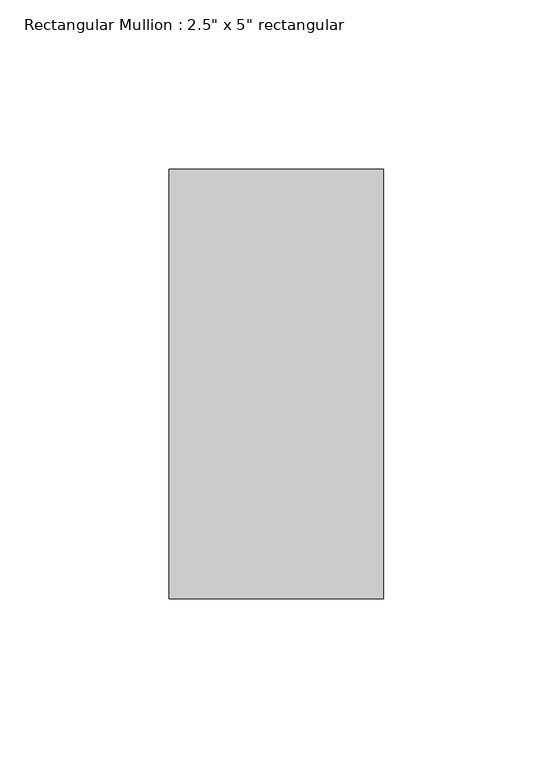
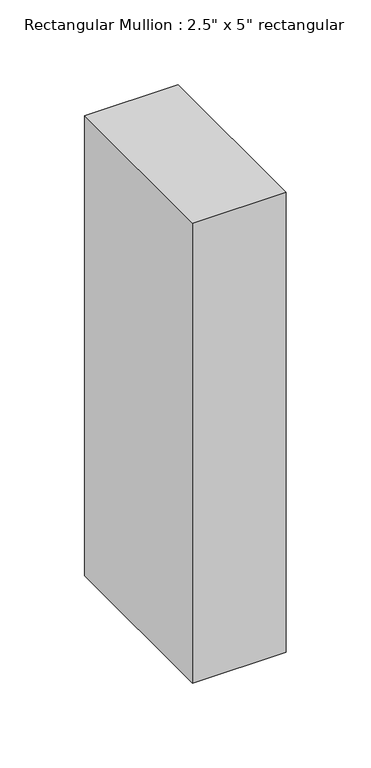
"""IFC4 building model written with IfcOpenShell, lengths in millimetres: member geometry."""

from ifc_helpers import new_model, si_unit, frame, origin, place, context, project, spatial, polyline, outline, extrude, source, transform, mapped, element, save


def member_0a8ab348(model_context):
    return source(origin(), model_context, "Body", "SweptSolid", [
        extrude(outline(polyline([(0.0, 63.5), (0.0, -63.5), (-63.5, -63.5), (-63.5, 63.5), (0.0, 63.5)])), frame((0.0, 0.0, -330.4597418), z_axis=(0.0, 0.0, 1.0), x_axis=(1.0, 0.0, 0.0)), (0.0, 0.0, 1.0), 330.4597418),
    ])


if __name__ == "__main__":
    model = new_model("IFC4")
    model_context = context("Model", 3, world=origin())
    ifc_project = project(units=[si_unit("LENGTHUNIT", "METRE", prefix="MILLI")], contexts=[model_context])
    site = spatial("IfcSite", under=ifc_project)
    building = spatial("IfcBuilding", under=site)
    placement = place(None, origin())
    member_shape = member_0a8ab348(model_context)
    element("IfcMember", 1, ObjectType="Rectangular Mullion : 2.5\" x 5\" rectangular", at=placement, inside=building, context=model_context, shape_type="MappedRepresentation", body=[
        mapped(member_shape, transform((0.0, 0.0, 0.0), x_axis=(1.0, 0.0, 0.0), y_axis=(0.0, 1.0, 0.0), z_axis=(0.0, 0.0, 1.0))),
    ])
    save(model, "model.ifc")

# Revit data of these elements
# Type "Rectangular Mullion : 2.5\" x 5\" rectangular"
#   built-in parameter 1007304 = 0.416667 (stored number, unit not read)
#   built-in parameter 1007301 = 0.104167 (stored number, unit not read)
#   built-in parameter 1007300 = 0.104167 (stored number, unit not read)
